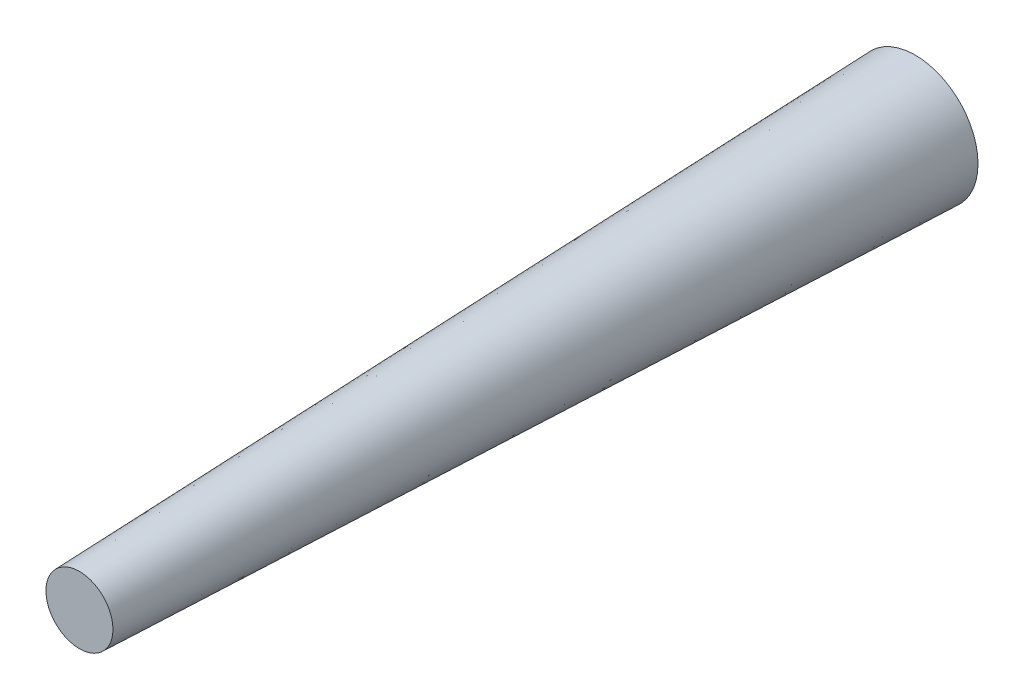
ISO-10303-21;
HEADER;
FILE_DESCRIPTION(('STEP AP214'),'2;1');
FILE_NAME('part.step','',(''),(''),'','','');
FILE_SCHEMA(('AUTOMOTIVE_DESIGN { 1 0 10303 214 1 1 1 1 }'));
ENDSEC;
DATA;
#1=APPLICATION_CONTEXT('core data for automotive mechanical design processes');
#2=APPLICATION_PROTOCOL_DEFINITION('international standard','automotive_design',2000,#1);
#3=PRODUCT_CONTEXT('',#1,'mechanical');
#4=PRODUCT('Part','Part','',(#3));
#5=PRODUCT_RELATED_PRODUCT_CATEGORY('part','',(#4));
#6=PRODUCT_DEFINITION_FORMATION('','',#4);
#7=PRODUCT_DEFINITION_CONTEXT('part definition',#1,'design');
#8=PRODUCT_DEFINITION('design','',#6,#7);
#9=PRODUCT_DEFINITION_SHAPE('','',#8);
#10=(LENGTH_UNIT() NAMED_UNIT(*) SI_UNIT(.MILLI.,.METRE.));
#11=(NAMED_UNIT(*) PLANE_ANGLE_UNIT() SI_UNIT($,.RADIAN.));
#12=(NAMED_UNIT(*) SI_UNIT($,.STERADIAN.) SOLID_ANGLE_UNIT());
#13=UNCERTAINTY_MEASURE_WITH_UNIT(LENGTH_MEASURE(1.E-05),#10,'distance_accuracy_value','');
#14=(GEOMETRIC_REPRESENTATION_CONTEXT(3) GLOBAL_UNCERTAINTY_ASSIGNED_CONTEXT((#13)) GLOBAL_UNIT_ASSIGNED_CONTEXT((#10,
#11,#12)) REPRESENTATION_CONTEXT('',''));
#15=CARTESIAN_POINT('',(0.,0.,0.));
#16=DIRECTION('',(0.,0.,1.));
#17=DIRECTION('',(1.,0.,0.));
#18=AXIS2_PLACEMENT_3D('',#15,#16,#17);
#19=CARTESIAN_POINT('',(0.,0.,0.));
#20=DIRECTION('',(0.,0.,-1.));
#21=DIRECTION('',(1.,0.,0.));
#22=AXIS2_PLACEMENT_3D('',#19,#20,#21);
#23=CONICAL_SURFACE('',#22,3.,0.0349065850398867);
#24=CARTESIAN_POINT('',(0.,0.,40.));
#25=DIRECTION('',(0.,0.,1.));
#26=DIRECTION('',(1.,0.,0.));
#27=AXIS2_PLACEMENT_3D('',#24,#25,#26);
#28=CIRCLE('',#27,1.60316922033009);
#29=CARTESIAN_POINT('',(1.60316922033009,0.,40.));
#30=VERTEX_POINT('',#29);
#31=EDGE_CURVE('E10',#30,#30,#28,.T.);
#32=ORIENTED_EDGE('',*,*,#31,.F.);
#33=EDGE_LOOP('',(#32));
#34=FACE_BOUND('',#33,.T.);
#35=CARTESIAN_POINT('',(0.,0.,0.));
#36=DIRECTION('',(0.,0.,1.));
#37=DIRECTION('',(1.,0.,0.));
#38=AXIS2_PLACEMENT_3D('',#35,#36,#37);
#39=CIRCLE('',#38,3.);
#40=CARTESIAN_POINT('',(3.,0.,0.));
#41=VERTEX_POINT('',#40);
#42=EDGE_CURVE('E43',#41,#41,#39,.T.);
#43=ORIENTED_EDGE('',*,*,#42,.T.);
#44=EDGE_LOOP('',(#43));
#45=FACE_BOUND('',#44,.T.);
#46=ADVANCED_FACE('F40',(#34,#45),#23,.T.);
#47=CARTESIAN_POINT('',(0.,0.,40.));
#48=DIRECTION('',(0.,0.,1.));
#49=DIRECTION('',(1.,0.,0.));
#50=AXIS2_PLACEMENT_3D('',#47,#48,#49);
#51=PLANE('',#50);
#52=ORIENTED_EDGE('',*,*,#31,.T.);
#53=EDGE_LOOP('',(#52));
#54=FACE_BOUND('',#53,.T.);
#55=ADVANCED_FACE('F55',(#54),#51,.T.);
#56=CARTESIAN_POINT('',(0.,0.,0.));
#57=DIRECTION('',(0.,0.,1.));
#58=DIRECTION('',(1.,0.,0.));
#59=AXIS2_PLACEMENT_3D('',#56,#57,#58);
#60=PLANE('',#59);
#61=ORIENTED_EDGE('',*,*,#42,.F.);
#62=EDGE_LOOP('',(#61));
#63=FACE_BOUND('',#62,.T.);
#64=ADVANCED_FACE('F49',(#63),#60,.F.);
#65=CLOSED_SHELL('',(#46,#55,#64));
#66=MANIFOLD_SOLID_BREP('B2',#65);
#67=ADVANCED_BREP_SHAPE_REPRESENTATION('',(#18,#66),#14);
#68=SHAPE_DEFINITION_REPRESENTATION(#9,#67);
ENDSEC;
END-ISO-10303-21;
